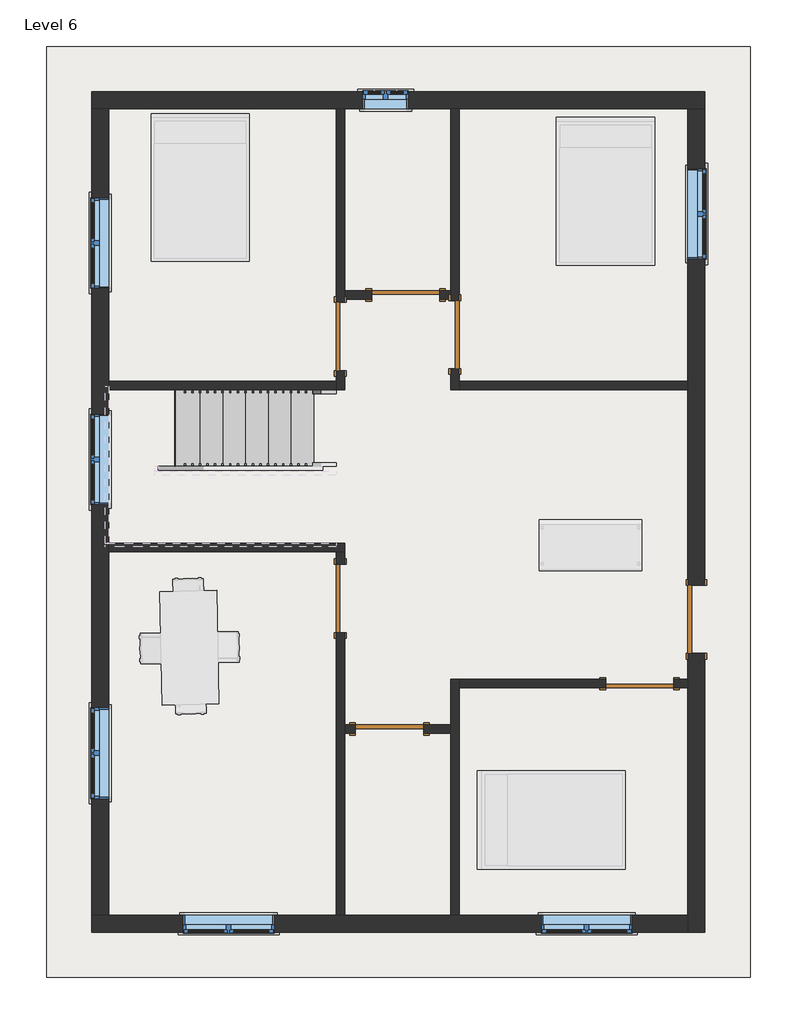
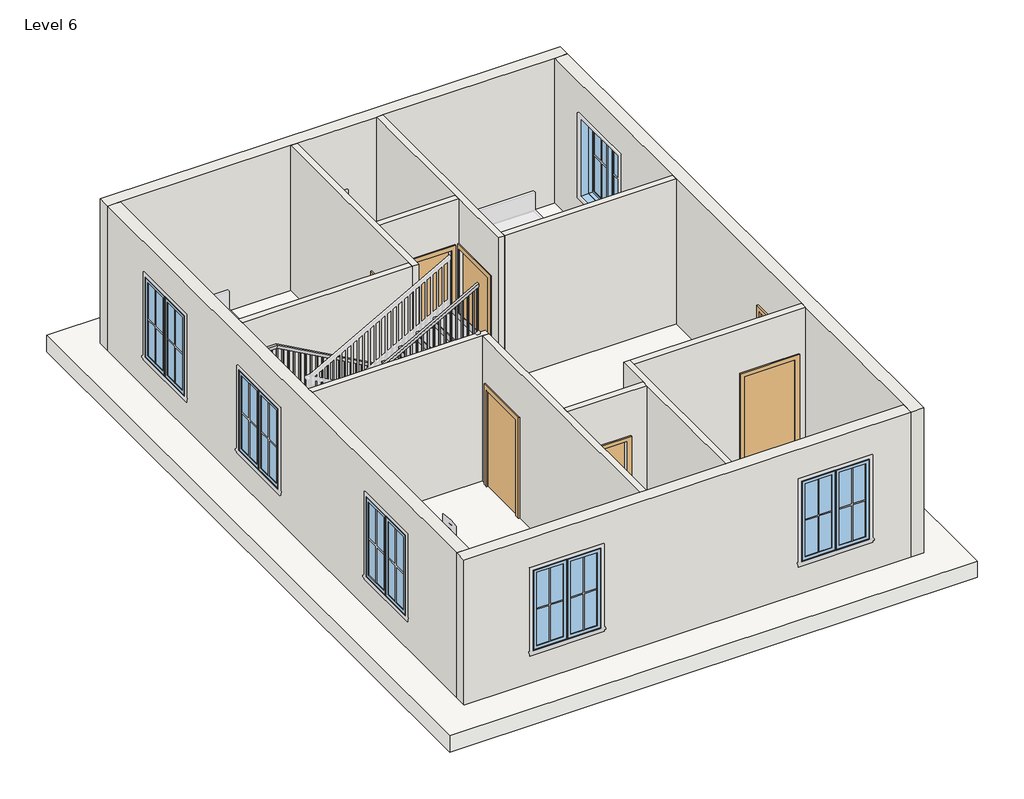
# One storey, part 1 of 2: 14 walls, 7 doors, 7 windows, 1 railing, 1 roof, 1 stair flight.
# Revit data of these elements (continued)
# Element 31 (IfcWindow, "Window-Casement-Double : 48\" x 60\"") (continued)
#   Phase Created = New Construction
#   Materials on its faces: "Wood - Stained", "Glass", "Clad - White"
# Materials
#   "Door - Panel": class "Wood", colour RGB 210 159 95, transparency 0, Cost = 0
#   "Door - Frame": colour RGB 118 70 51, transparency 0, Cost = 0
#   "Wood - Stained": class "Wood", colour RGB 224 178 126, transparency 0, Cost = 0
#   "Glass": class "Glass", colour RGB 0 128 192, transparency 0.75, Description = "Soda Lime Glass", Cost = 0
#   "Clad - White": class "Wood", colour RGB 242 242 238, transparency 0, Cost = 0
#   "Flor_Branco": class "Paint", colour RGB 255 255 255, transparency 0
#   "Default Roof": colour RGB 88 101 114, transparency 0, Cost = 0
#   "Default Wall": colour RGB 128 128 128, transparency 0, Cost = 0
#   "Sash": class "Wood", colour RGB 224 178 126, transparency 0, Cost = 0
